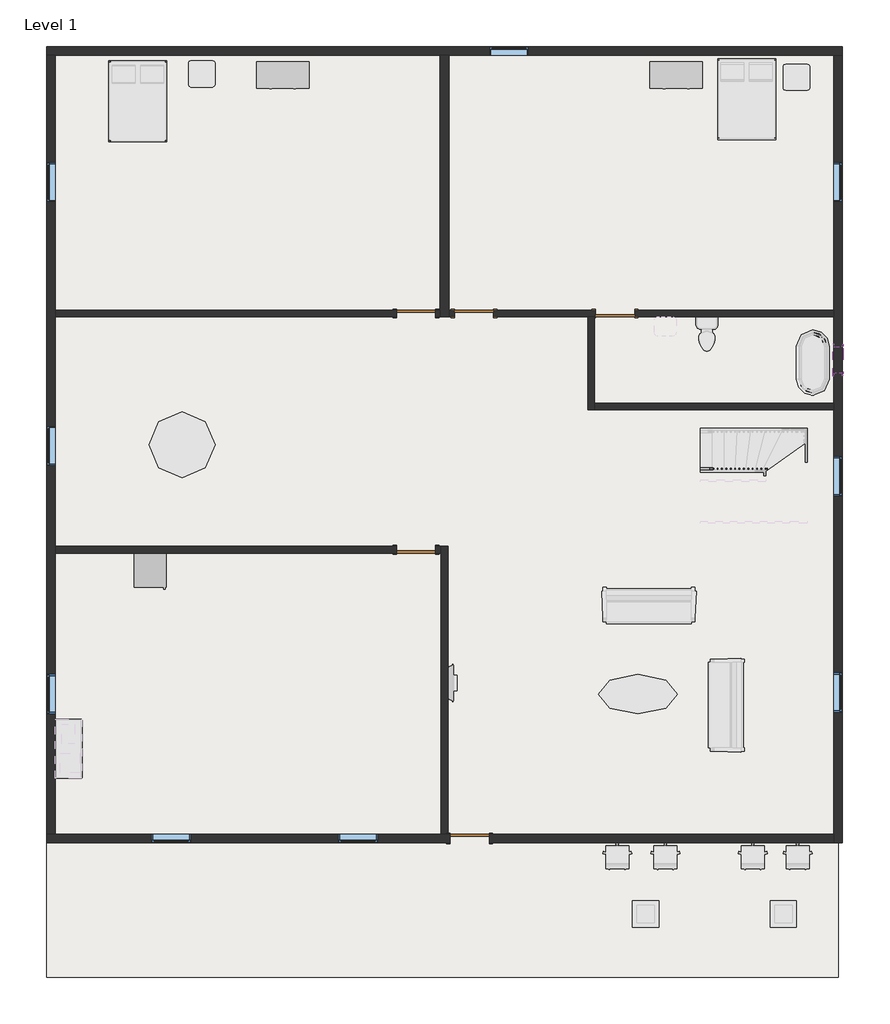
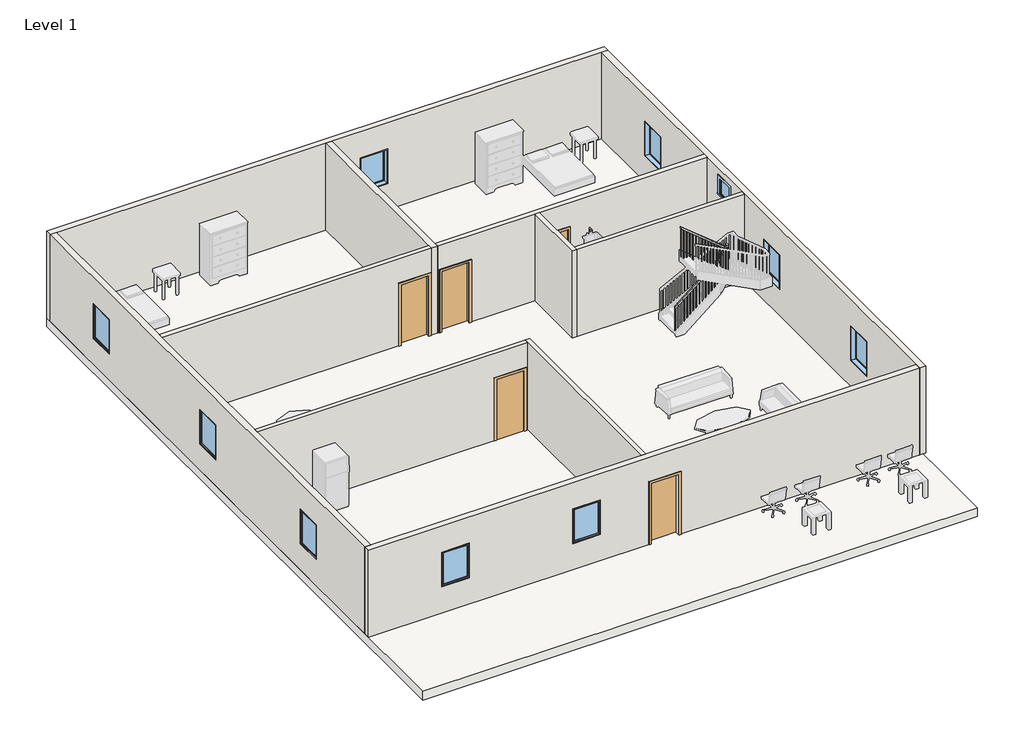
# One storey, part 1 of 2: 11 walls, 10 windows, 5 doors, 1 railing, 1 slab.
"""IFC4 building model written with IfcOpenShell, lengths in millimetres."""

from ifc_helpers import new_model, si_unit, frame, origin, origin_with_axes, place, context, project, spatial, polyline, outline, extrude, faceted_brep, transform, mapped, element, save
from components import door_16372e1c, door_686f89d2, door_719f80de, window_e2841890, window_e41d21a6

model = new_model("IFC4")

# Units and contexts
model_context = context("Model", 3, world=origin())
ifc_project = project(units=[si_unit("LENGTHUNIT", "METRE", prefix="MILLI")], contexts=[model_context])

# Site, building, storey
site = spatial("IfcSite", under=ifc_project)
building = spatial("IfcBuilding", under=site)
storey = spatial("IfcBuildingStorey", under=building, Name="Level 1", Elevation=0.0)

# Doors
placement = place(None, origin())
door_shape = door_16372e1c(model_context)
element("IfcDoor", 1, ObjectType="Single-Flush : 36\" x 84\"", at=placement, inside=storey, context=model_context, shape_type="MappedRepresentation", body=[
    mapped(door_shape, transform((-8051.9808972, 8246.1716937, 0.0), x_axis=(1.0, 0.0, 0.0), y_axis=(0.0, 1.0, 0.0), z_axis=(0.0, 0.0, 1.0))),
])
element("IfcDoor", 2, ObjectType="Single-Flush : 36\" x 84\"", at=placement, inside=storey, context=model_context, shape_type="MappedRepresentation", body=[
    mapped(door_shape, transform((-3429.1808972, 8246.1716937, 0.0), x_axis=(-1.0, 0.0, 0.0), y_axis=(0.0, -1.0, 0.0), z_axis=(0.0, 0.0, 1.0))),
])
door_2_shape = door_686f89d2(model_context)
element("IfcDoor", 3, ObjectType="Single-Flush : 36\" x 84\"", at=placement, inside=storey, context=model_context, shape_type="MappedRepresentation", body=[
    mapped(door_2_shape, transform((-6705.7808972, 8246.1716937, 0.0), x_axis=(-1.0, 0.0, 0.0), y_axis=(0.0, -1.0, 0.0), z_axis=(0.0, 0.0, 1.0))),
])
element("IfcDoor", 4, ObjectType="Single-Flush : 36\" x 84\"", at=placement, inside=storey, context=model_context, shape_type="MappedRepresentation", body=[
    mapped(door_2_shape, transform((-8051.9808972, 2759.7716937, 0.0), x_axis=(1.0, 0.0, 0.0), y_axis=(0.0, 1.0, 0.0), z_axis=(0.0, 0.0, 1.0))),
])
door_3_shape = door_719f80de(model_context)
element("IfcDoor", 5, ObjectType="Single-Flush : 36\" x 84\"", at=placement, inside=storey, context=model_context, shape_type="MappedRepresentation", body=[
    mapped(door_3_shape, transform((-6807.3808972, -3945.8283063, 0.0), x_axis=(-1.0, 0.0, 0.0), y_axis=(0.0, -1.0, 0.0), z_axis=(0.0, 0.0, 1.0))),
])

# Railing
element("IfcRailing", 6, ObjectType="Handrail - Rectangular", at=placement, inside=storey, context=model_context, shape_type="SolidModel", body=[
    faceted_brep([(-1451.7125891, 4664.7716937, 1025.2529681), (-1451.7125891, 4664.7716937, 959.7067088), (-1451.7125891, 4613.9716937, 959.7067088), (-1451.7125891, 4613.9716937, 1025.2529681), (-0.1808972, 4664.7716937, 2208.7848338), (50.6191028, 4664.7716937, 2184.659247), (50.6191028, 4613.9716937, 2184.659247), (-0.1808972, 4613.9716937, 2208.7848338), (-0.1808972, 4664.7716937, 2414.6281882), (50.6191028, 4664.7716937, 2363.8281882), (50.6191028, 4613.9716937, 2363.8281882), (-0.1808972, 4613.9716937, 2414.6281882), (126.8191028, 4664.7716937, 2414.6281882), (126.8191028, 4664.7716937, 2363.8281882), (76.0191028, 4613.9716937, 2363.8281882), (76.0191028, 4613.9716937, 2414.6281882), (126.8191028, 4537.7716937, 2414.6281882), (126.8191028, 4508.6503599, 2363.8281882), (76.0191028, 4508.6503599, 2363.8281882), (76.0191028, 4537.7716937, 2414.6281882), (126.8191028, 4410.7716937, 2631.5051451), (126.8191028, 4359.9716937, 2617.7256424), (76.0191028, 4359.9716937, 2617.7256424), (76.0191028, 4410.7716937, 2631.5051451), (126.8191028, 4410.7716937, 2837.3484995), (126.8191028, 4359.9716937, 2786.5484995), (76.0191028, 4359.9716937, 2786.5484995), (76.0191028, 4410.7716937, 2837.3484995), (126.8191028, 4283.7716937, 2837.3484995), (126.8191028, 4283.7716937, 2786.5484995), (76.0191028, 4334.5716937, 2786.5484995), (76.0191028, 4334.5716937, 2837.3484995), (-0.1808972, 4283.7716937, 2837.3484995), (-18.2663103, 4283.7716937, 2786.5484995), (-18.2663103, 4334.5716937, 2786.5484995), (-0.1808972, 4334.5716937, 2837.3484995), (-1451.7125891, 4283.7716937, 4020.8803652), (-1451.7125891, 4334.5716937, 4020.8803652), (-1451.7125891, 4334.5716937, 3955.3341059), (-1451.7125891, 4283.7716937, 3955.3341059)], [[[0, 1, 2, 3]], [[1, 0, 4, 5]], [[2, 1, 5, 6]], [[3, 2, 6, 7]], [[0, 3, 7, 4]], [[5, 4, 8, 9]], [[6, 5, 9, 10]], [[7, 6, 10, 11]], [[4, 7, 11, 8]], [[9, 8, 12, 13]], [[10, 9, 13, 14]], [[11, 10, 14, 15]], [[8, 11, 15, 12]], [[13, 12, 16, 17]], [[14, 13, 17, 18]], [[15, 14, 18, 19]], [[12, 15, 19, 16]], [[17, 16, 20, 21]], [[18, 17, 21, 22]], [[19, 18, 22, 23]], [[16, 19, 23, 20]], [[21, 20, 24, 25]], [[22, 21, 25, 26]], [[23, 22, 26, 27]], [[20, 23, 27, 24]], [[25, 24, 28, 29]], [[26, 25, 29, 30]], [[27, 26, 30, 31]], [[24, 27, 31, 28]], [[29, 28, 32, 33]], [[30, 29, 33, 34]], [[31, 30, 34, 35]], [[28, 31, 35, 32]], [[36, 37, 38, 39]], [[33, 32, 36, 39]], [[34, 33, 39, 38]], [[35, 34, 38, 37]], [[32, 35, 37, 36]]]),
    extrude(outline(polyline([(3866.2231262, -1342.4232536), (3881.7558784, -1361.4732536), (2878.6666667, -1361.4732536), (2878.6666667, -1342.4232536), (3866.2231262, -1342.4232536)])), frame((0.0, 4299.6466937, 0.0), z_axis=(0.0, 1.0, 0.0), x_axis=(0.0, 0.0, 1.0)), (0.0, 0.0, 1.0), 19.05),
    extrude(outline(polyline([(3783.3817813, -1240.8232536), (3798.9145334, -1259.8732536), (2878.6666667, -1259.8732536), (2878.6666667, -1240.8232536), (3783.3817813, -1240.8232536)])), frame((0.0, 4299.6466937, 0.0), z_axis=(0.0, 1.0, 0.0), x_axis=(0.0, 0.0, 1.0)), (0.0, 0.0, 1.0), 19.05),
    extrude(outline(polyline([(3700.5404364, -1139.2232536), (3716.0731885, -1158.2732536), (2709.3333333, -1158.2732536), (2709.3333333, -1139.2232536), (3700.5404364, -1139.2232536)])), frame((0.0, 4299.6466937, 0.0), z_axis=(0.0, 1.0, 0.0), x_axis=(0.0, 0.0, 1.0)), (0.0, 0.0, 1.0), 19.05),
    extrude(outline(polyline([(3617.6990914, -1037.6232536), (3633.2318436, -1056.6732536), (2709.3333333, -1056.6732536), (2709.3333333, -1037.6232536), (3617.6990914, -1037.6232536)])), frame((0.0, 4299.6466937, 0.0), z_axis=(0.0, 1.0, 0.0), x_axis=(0.0, 0.0, 1.0)), (0.0, 0.0, 1.0), 19.05),
    extrude(outline(polyline([(3534.8577465, -936.0232536), (3550.3904987, -955.0732536), (2709.3333333, -955.0732536), (2709.3333333, -936.0232536), (3534.8577465, -936.0232536)])), frame((0.0, 4299.6466937, 0.0), z_axis=(0.0, 1.0, 0.0), x_axis=(0.0, 0.0, 1.0)), (0.0, 0.0, 1.0), 19.05),
    extrude(outline(polyline([(3452.0164016, -834.4232536), (3467.5491538, -853.4732536), (2540.0, -853.4732536), (2540.0, -834.4232536), (3452.0164016, -834.4232536)])), frame((0.0, 4299.6466937, 0.0), z_axis=(0.0, 1.0, 0.0), x_axis=(0.0, 0.0, 1.0)), (0.0, 0.0, 1.0), 19.05),
    extrude(outline(polyline([(3369.1750567, -732.8232536), (3384.7078088, -751.8732536), (2540.0, -751.8732536), (2540.0, -732.8232536), (3369.1750567, -732.8232536)])), frame((0.0, 4299.6466937, 0.0), z_axis=(0.0, 1.0, 0.0), x_axis=(0.0, 0.0, 1.0)), (0.0, 0.0, 1.0), 19.05),
    extrude(outline(polyline([(3286.3337117, -631.2232536), (3301.8664639, -650.2732536), (2540.0, -650.2732536), (2540.0, -631.2232536), (3286.3337117, -631.2232536)])), frame((0.0, 4299.6466937, 0.0), z_axis=(0.0, 1.0, 0.0), x_axis=(0.0, 0.0, 1.0)), (0.0, 0.0, 1.0), 19.05),
    extrude(outline(polyline([(3203.4923668, -529.6232536), (3219.025119, -548.6732536), (2370.6666667, -548.6732536), (2370.6666667, -529.6232536), (3203.4923668, -529.6232536)])), frame((0.0, 4299.6466937, 0.0), z_axis=(0.0, 1.0, 0.0), x_axis=(0.0, 0.0, 1.0)), (0.0, 0.0, 1.0), 19.05),
    extrude(outline(polyline([(3120.6510219, -428.0232536), (3136.1837741, -447.0732536), (2370.6666667, -447.0732536), (2370.6666667, -428.0232536), (3120.6510219, -428.0232536)])), frame((0.0, 4299.6466937, 0.0), z_axis=(0.0, 1.0, 0.0), x_axis=(0.0, 0.0, 1.0)), (0.0, 0.0, 1.0), 19.05),
    extrude(outline(polyline([(3037.809677, -326.4232536), (3053.3424291, -345.4732536), (2201.3333333, -345.4732536), (2201.3333333, -326.4232536), (3037.809677, -326.4232536)])), frame((0.0, 4299.6466937, 0.0), z_axis=(0.0, 1.0, 0.0), x_axis=(0.0, 0.0, 1.0)), (0.0, 0.0, 1.0), 19.05),
    extrude(outline(polyline([(2954.9683321, -224.8232536), (2970.5010842, -243.8732536), (2201.3333333, -243.8732536), (2201.3333333, -224.8232536), (2954.9683321, -224.8232536)])), frame((0.0, 4299.6466937, 0.0), z_axis=(0.0, 1.0, 0.0), x_axis=(0.0, 0.0, 1.0)), (0.0, 0.0, 1.0), 19.05),
    extrude(outline(polyline([(2872.1269871, -123.2232536), (2887.6597393, -142.2732536), (2032.0, -142.2732536), (2032.0, -123.2232536), (2872.1269871, -123.2232536)])), frame((0.0, 4299.6466937, 0.0), z_axis=(0.0, 1.0, 0.0), x_axis=(0.0, 0.0, 1.0)), (0.0, 0.0, 1.0), 19.05),
    extrude(outline(polyline([(2789.2856422, -21.6232536), (2804.8183944, -40.6732536), (2032.0, -40.6732536), (2032.0, -21.6232536), (2789.2856422, -21.6232536)])), frame((0.0, 4299.6466937, 0.0), z_axis=(0.0, 1.0, 0.0), x_axis=(0.0, 0.0, 1.0)), (0.0, 0.0, 1.0), 19.05),
    extrude(outline(polyline([(4411.86079, 2529.115018), (4430.91079, 2496.5834745), (4430.91079, 1524.0), (4411.86079, 1524.0), (4411.86079, 2529.115018)])), frame((91.8941028, 0.0, 0.0), z_axis=(1.0, 0.0, 0.0), x_axis=(0.0, 1.0, 0.0)), (0.0, 0.0, 1.0), 19.05),
    extrude(outline(polyline([(4513.46079, 2355.6134525), (4532.51079, 2323.0819089), (4532.51079, 1524.0), (4513.46079, 1524.0), (4513.46079, 2355.6134525)])), frame((91.8941028, 0.0, 0.0), z_axis=(1.0, 0.0, 0.0), x_axis=(0.0, 1.0, 0.0)), (0.0, 0.0, 1.0), 19.05),
    extrude(outline(polyline([(2127.2519138, -19.7875891), (2111.7191617, -38.8375891), (1016.0, -38.8375891), (1016.0, -19.7875891), (2127.2519138, -19.7875891)])), frame((0.0, 4629.8466937, 0.0), z_axis=(0.0, 1.0, 0.0), x_axis=(0.0, 0.0, 1.0)), (0.0, 0.0, 1.0), 19.05),
    extrude(outline(polyline([(2044.4105689, -121.3875891), (2028.8778167, -140.4375891), (1016.0, -140.4375891), (1016.0, -121.3875891), (2044.4105689, -121.3875891)])), frame((0.0, 4629.8466937, 0.0), z_axis=(0.0, 1.0, 0.0), x_axis=(0.0, 0.0, 1.0)), (0.0, 0.0, 1.0), 19.05),
    extrude(outline(polyline([(1961.569224, -222.9875891), (1946.0364718, -242.0375891), (846.6666667, -242.0375891), (846.6666667, -222.9875891), (1961.569224, -222.9875891)])), frame((0.0, 4629.8466937, 0.0), z_axis=(0.0, 1.0, 0.0), x_axis=(0.0, 0.0, 1.0)), (0.0, 0.0, 1.0), 19.05),
    extrude(outline(polyline([(1878.7278791, -324.5875891), (1863.1951269, -343.6375891), (846.6666667, -343.6375891), (846.6666667, -324.5875891), (1878.7278791, -324.5875891)])), frame((0.0, 4629.8466937, 0.0), z_axis=(0.0, 1.0, 0.0), x_axis=(0.0, 0.0, 1.0)), (0.0, 0.0, 1.0), 19.05),
    extrude(outline(polyline([(1795.8865341, -426.1875891), (1780.353782, -445.2375891), (677.3333333, -445.2375891), (677.3333333, -426.1875891), (1795.8865341, -426.1875891)])), frame((0.0, 4629.8466937, 0.0), z_axis=(0.0, 1.0, 0.0), x_axis=(0.0, 0.0, 1.0)), (0.0, 0.0, 1.0), 19.05),
    extrude(outline(polyline([(1713.0451892, -527.7875891), (1697.5124371, -546.8375891), (677.3333333, -546.8375891), (677.3333333, -527.7875891), (1713.0451892, -527.7875891)])), frame((0.0, 4629.8466937, 0.0), z_axis=(0.0, 1.0, 0.0), x_axis=(0.0, 0.0, 1.0)), (0.0, 0.0, 1.0), 19.05),
    extrude(outline(polyline([(1630.2038443, -629.3875891), (1614.6710921, -648.4375891), (508.0, -648.4375891), (508.0, -629.3875891), (1630.2038443, -629.3875891)])), frame((0.0, 4629.8466937, 0.0), z_axis=(0.0, 1.0, 0.0), x_axis=(0.0, 0.0, 1.0)), (0.0, 0.0, 1.0), 19.05),
    extrude(outline(polyline([(1547.3624994, -730.9875891), (1531.8297472, -750.0375891), (508.0, -750.0375891), (508.0, -730.9875891), (1547.3624994, -730.9875891)])), frame((0.0, 4629.8466937, 0.0), z_axis=(0.0, 1.0, 0.0), x_axis=(0.0, 0.0, 1.0)), (0.0, 0.0, 1.0), 19.05),
    extrude(outline(polyline([(1464.5211545, -832.5875891), (1448.9884023, -851.6375891), (508.0, -851.6375891), (508.0, -832.5875891), (1464.5211545, -832.5875891)])), frame((0.0, 4629.8466937, 0.0), z_axis=(0.0, 1.0, 0.0), x_axis=(0.0, 0.0, 1.0)), (0.0, 0.0, 1.0), 19.05),
    extrude(outline(polyline([(1381.6798095, -934.1875891), (1366.1470574, -953.2375891), (338.6666667, -953.2375891), (338.6666667, -934.1875891), (1381.6798095, -934.1875891)])), frame((0.0, 4629.8466937, 0.0), z_axis=(0.0, 1.0, 0.0), x_axis=(0.0, 0.0, 1.0)), (0.0, 0.0, 1.0), 19.05),
    extrude(outline(polyline([(1298.8384646, -1035.7875891), (1283.3057124, -1054.8375891), (338.6666667, -1054.8375891), (338.6666667, -1035.7875891), (1298.8384646, -1035.7875891)])), frame((0.0, 4629.8466937, 0.0), z_axis=(0.0, 1.0, 0.0), x_axis=(0.0, 0.0, 1.0)), (0.0, 0.0, 1.0), 19.05),
    extrude(outline(polyline([(1215.9971197, -1137.3875891), (1200.4643675, -1156.4375891), (338.6666667, -1156.4375891), (338.6666667, -1137.3875891), (1215.9971197, -1137.3875891)])), frame((0.0, 4629.8466937, 0.0), z_axis=(0.0, 1.0, 0.0), x_axis=(0.0, 0.0, 1.0)), (0.0, 0.0, 1.0), 19.05),
    extrude(outline(polyline([(1133.1557748, -1238.9875891), (1117.6230226, -1258.0375891), (169.3333333, -1258.0375891), (169.3333333, -1238.9875891), (1133.1557748, -1238.9875891)])), frame((0.0, 4629.8466937, 0.0), z_axis=(0.0, 1.0, 0.0), x_axis=(0.0, 0.0, 1.0)), (0.0, 0.0, 1.0), 19.05),
    extrude(outline(polyline([(1050.3144298, -1340.5875891), (1034.7816777, -1359.6375891), (169.3333333, -1359.6375891), (169.3333333, -1340.5875891), (1050.3144298, -1340.5875891)])), frame((0.0, 4629.8466937, 0.0), z_axis=(0.0, 1.0, 0.0), x_axis=(0.0, 0.0, 1.0)), (0.0, 0.0, 1.0), 19.05),
    extrude(outline(polyline([(79.9767464, 4318.6966937), (79.9767464, 4299.6466937), (60.9267464, 4299.6466937), (60.9267464, 4318.6966937), (79.9767464, 4318.6966937)])), frame((0.0, 0.0, 1862.6666667), z_axis=(0.0, 0.0, 1.0), x_axis=(1.0, 0.0, 0.0)), (0.0, 0.0, 1.0), 923.8818329),
    extrude(outline(polyline([(91.8941028, 4318.6966937), (110.9441028, 4318.6966937), (110.9441028, 4299.6466937), (91.8941028, 4299.6466937), (91.8941028, 4318.6966937)])), frame((0.0, 0.0, 1862.6666667), z_axis=(0.0, 0.0, 1.0), x_axis=(1.0, 0.0, 0.0)), (0.0, 0.0, 1.0), 923.8818329),
    extrude(outline(polyline([(91.8941028, 4333.4825975), (110.9441028, 4333.4825975), (110.9441028, 4314.4325975), (91.8941028, 4314.4325975), (91.8941028, 4333.4825975)])), frame((0.0, 0.0, 1693.3333333), z_axis=(0.0, 0.0, 1.0), x_axis=(1.0, 0.0, 0.0)), (0.0, 0.0, 1.0), 1093.2151662),
    extrude(outline(polyline([(91.8941028, 4634.11079), (110.9441028, 4634.11079), (110.9441028, 4615.06079), (91.8941028, 4615.06079), (91.8941028, 4634.11079)])), frame((0.0, 0.0, 1354.6666667), z_axis=(0.0, 0.0, 1.0), x_axis=(1.0, 0.0, 0.0)), (0.0, 0.0, 1.0), 1009.1615215),
    extrude(outline(polyline([(91.8941028, 4629.8466937), (91.8941028, 4648.8966937), (110.9441028, 4648.8966937), (110.9441028, 4629.8466937), (91.8941028, 4629.8466937)])), frame((0.0, 0.0, 1185.3333333), z_axis=(0.0, 0.0, 1.0), x_axis=(1.0, 0.0, 0.0)), (0.0, 0.0, 1.0), 1178.4948549),
    extrude(outline(polyline([(60.9267464, 4629.8466937), (60.9267464, 4648.8966937), (79.9767464, 4648.8966937), (79.9767464, 4629.8466937), (60.9267464, 4629.8466937)])), frame((0.0, 0.0, 1185.3333333), z_axis=(0.0, 0.0, 1.0), x_axis=(1.0, 0.0, 0.0)), (0.0, 0.0, 1.0), 1178.4948549),
    extrude(outline(polyline([(3939.8013537, -1432.6625891), (3955.3341059, -1451.7125891), (2878.6666667, -1451.7125891), (2878.6666667, -1432.6625891), (3939.8013537, -1432.6625891)])), frame((0.0, 4299.6466937, 0.0), z_axis=(0.0, 1.0, 0.0), x_axis=(0.0, 0.0, 1.0)), (0.0, 0.0, 1.0), 19.05),
    extrude(outline(polyline([(975.239461, -1432.6625891), (959.7067088, -1451.7125891), (169.3333333, -1451.7125891), (169.3333333, -1432.6625891), (975.239461, -1432.6625891)])), frame((0.0, 4629.8466937, 0.0), z_axis=(0.0, 1.0, 0.0), x_axis=(0.0, 0.0, 1.0)), (0.0, 0.0, 1.0), 19.05),
])

# Slab
element("IfcSlab", 7, ObjectType="Generic - 12\"", at=placement, inside=storey, context=model_context, shape_type="SweptSolid", body=[
    extrude(outline(polyline([(1761.9441028, 14443.7716937), (1761.9441028, -7171.6283063), (-16637.1808972, -7171.6283063), (-16637.1808972, 14443.7716937), (1761.9441028, 14443.7716937)])), frame((0.0, 0.0, -304.8), z_axis=(0.0, 0.0, 1.0), x_axis=(1.0, 0.0, 0.0)), (0.0, 0.0, 1.0), 304.8),
])

# Walls
element("IfcWall", 8, ObjectType="Generic - 8\"", at=placement, inside=storey, context=model_context, shape_type="Brep", body=[
    faceted_brep([(-16637.1808972, 14240.5716937, 0.0), (-16433.9808972, 14240.5716937, 0.0), (-7493.1808972, 14240.5716937, 0.0), (-7289.9808972, 14240.5716937, 0.0), (1650.8191028, 14240.5716937, 0.0), (1854.0191028, 14240.5716937, 0.0), (1854.0191028, 14240.5716937, 3048.0), (1650.8191028, 14240.5716937, 3048.0), (-7289.9808972, 14240.5716937, 3048.0), (-7493.1808972, 14240.5716937, 3048.0), (-16433.9808972, 14240.5716937, 3048.0), (-16637.1808972, 14240.5716937, 3048.0), (-5435.7808972, 14240.5716937, 2133.6), (-5435.7808972, 14240.5716937, 914.4), (-6350.1808972, 14240.5716937, 914.4), (-6350.1808972, 14240.5716937, 2133.6), (-16637.1808972, 14443.7716937, 0.0), (-16637.1808972, 14443.7716937, 3048.0), (1854.0191028, 14443.7716937, 3048.0), (1854.0191028, 14443.7716937, 0.0), (-5435.7808972, 14443.7716937, 2133.6), (-6350.1808972, 14443.7716937, 2133.6), (-6350.1808972, 14443.7716937, 914.4), (-5435.7808972, 14443.7716937, 914.4)], [[[0, 1, 2, 3, 4, 5, 6, 7, 8, 9, 10, 11], [12, 13, 14, 15]], [[16, 17, 18, 19], [20, 21, 22, 23]], [[5, 4, 3, 2, 1, 0, 16, 19]], [[11, 10, 9, 8, 7, 6, 18, 17]], [[6, 5, 19, 18]], [[0, 11, 17, 16]], [[13, 12, 20, 23]], [[14, 13, 23, 22]], [[15, 14, 22, 21]], [[12, 15, 21, 20]]]),
])
element("IfcWall", 9, ObjectType="Generic - 8\"", at=placement, inside=storey, context=model_context, shape_type="Brep", body=[
    faceted_brep([(1650.8191028, 14240.5716937, 0.0), (1650.8191028, 8322.3716937, 0.0), (1650.8191028, 8169.9716937, 0.0), (1650.8191028, 6163.3716937, 0.0), (1650.8191028, 6010.9716937, 0.0), (1650.8191028, -3844.2283063, 0.0), (1650.8191028, -4047.4283063, 0.0), (1650.8191028, -4047.4283063, 3048.0), (1650.8191028, -3844.2283063, 3048.0), (1650.8191028, 6010.9716937, 3048.0), (1650.8191028, 6163.3716937, 3048.0), (1650.8191028, 8169.9716937, 3048.0), (1650.8191028, 8322.3716937, 3048.0), (1650.8191028, 14240.5716937, 3048.0), (1650.8191028, -1008.9533063, 2133.6), (1650.8191028, -1008.9533063, 914.4), (1650.8191028, -94.5533063, 914.4), (1650.8191028, -94.5533063, 2133.6), (1650.8191028, 4007.5466937, 2133.6), (1650.8191028, 4007.5466937, 914.4), (1650.8191028, 4921.9466937, 914.4), (1650.8191028, 4921.9466937, 2133.6), (1650.8191028, 10836.9716937, 2133.6), (1650.8191028, 10836.9716937, 914.4), (1650.8191028, 11751.3716937, 914.4), (1650.8191028, 11751.3716937, 2133.6), (1650.8191028, 7471.4716937, 2768.6), (1650.8191028, 6861.8716937, 2768.6), (1650.8191028, 6861.8716937, 2159.0), (1650.8191028, 7471.4716937, 2159.0), (1854.0191028, 14240.5716937, 0.0), (1854.0191028, 14240.5716937, 3048.0), (1854.0191028, -4047.4283063, 3048.0), (1854.0191028, -4047.4283063, 0.0), (1854.0191028, -1008.9533063, 2133.6), (1854.0191028, -94.5533063, 2133.6), (1854.0191028, -94.5533063, 914.4), (1854.0191028, -1008.9533063, 914.4), (1854.0191028, 4007.5466937, 2133.6), (1854.0191028, 4921.9466937, 2133.6), (1854.0191028, 4921.9466937, 914.4), (1854.0191028, 4007.5466937, 914.4), (1854.0191028, 10836.9716937, 2133.6), (1854.0191028, 11751.3716937, 2133.6), (1854.0191028, 11751.3716937, 914.4), (1854.0191028, 10836.9716937, 914.4), (1854.0191028, 7471.4716937, 2768.6), (1854.0191028, 7471.4716937, 2159.0), (1854.0191028, 6861.8716937, 2159.0), (1854.0191028, 6861.8716937, 2768.6)], [[[0, 1, 2, 3, 4, 5, 6, 7, 8, 9, 10, 11, 12, 13], [14, 15, 16, 17], [18, 19, 20, 21], [22, 23, 24, 25], [26, 27, 28, 29]], [[30, 31, 32, 33], [34, 35, 36, 37], [38, 39, 40, 41], [42, 43, 44, 45], [46, 47, 48, 49]], [[6, 5, 4, 3, 2, 1, 0, 30, 33]], [[13, 12, 11, 10, 9, 8, 7, 32, 31]], [[0, 13, 31, 30]], [[7, 6, 33, 32]], [[15, 14, 34, 37]], [[16, 15, 37, 36]], [[17, 16, 36, 35]], [[14, 17, 35, 34]], [[19, 18, 38, 41]], [[20, 19, 41, 40]], [[21, 20, 40, 39]], [[18, 21, 39, 38]], [[23, 22, 42, 45]], [[24, 23, 45, 44]], [[25, 24, 44, 43]], [[22, 25, 43, 42]], [[47, 46, 26, 29]], [[48, 47, 29, 28]], [[49, 48, 28, 27]], [[46, 49, 27, 26]]]),
])
element("IfcWall", 10, ObjectType="Generic - 8\"", at=placement, inside=storey, context=model_context, shape_type="Brep", body=[
    faceted_brep([(-7264.5808972, -3844.2283063, 2133.6), (-7264.5808972, -3844.2283063, 0.0), (-7315.3808972, -3844.2283063, 0.0), (-7467.7808972, -3844.2283063, 0.0), (-16433.9808972, -3844.2283063, 0.0), (-16637.1808972, -3844.2283063, 0.0), (-16637.1808972, -3844.2283063, 3048.0), (-16433.9808972, -3844.2283063, 3048.0), (-7467.7808972, -3844.2283063, 3048.0), (-7315.3808972, -3844.2283063, 3048.0), (1650.8191028, -3844.2283063, 3048.0), (1650.8191028, -3844.2283063, 0.0), (-6350.1808972, -3844.2283063, 0.0), (-6350.1808972, -3844.2283063, 2133.6), (-14198.7808972, -3844.2283063, 2133.6), (-14198.7808972, -3844.2283063, 914.4), (-13284.3808972, -3844.2283063, 914.4), (-13284.3808972, -3844.2283063, 2133.6), (-9855.3808972, -3844.2283063, 2133.6), (-9855.3808972, -3844.2283063, 914.4), (-8940.9808972, -3844.2283063, 914.4), (-8940.9808972, -3844.2283063, 2133.6), (-16637.1808972, -4047.4283063, 0.0), (-7264.5808972, -4047.4283063, 0.0), (-7264.5808972, -4047.4283063, 2133.6), (-6350.1808972, -4047.4283063, 2133.6), (-6350.1808972, -4047.4283063, 0.0), (1650.8191028, -4047.4283063, 0.0), (1650.8191028, -4047.4283063, 3048.0), (-16637.1808972, -4047.4283063, 3048.0), (-14198.7808972, -4047.4283063, 2133.6), (-13284.3808972, -4047.4283063, 2133.6), (-13284.3808972, -4047.4283063, 914.4), (-14198.7808972, -4047.4283063, 914.4), (-9855.3808972, -4047.4283063, 2133.6), (-8940.9808972, -4047.4283063, 2133.6), (-8940.9808972, -4047.4283063, 914.4), (-9855.3808972, -4047.4283063, 914.4)], [[[0, 1, 2, 3, 4, 5, 6, 7, 8, 9, 10, 11, 12, 13], [14, 15, 16, 17], [18, 19, 20, 21]], [[22, 23, 24, 25, 26, 27, 28, 29], [30, 31, 32, 33], [34, 35, 36, 37]], [[12, 11, 27, 26]], [[5, 4, 3, 2, 1, 23, 22]], [[10, 9, 8, 7, 6, 29, 28]], [[11, 10, 28, 27]], [[6, 5, 22, 29]], [[24, 23, 1, 0]], [[25, 24, 0, 13]], [[26, 25, 13, 12]], [[15, 14, 30, 33]], [[16, 15, 33, 32]], [[17, 16, 32, 31]], [[14, 17, 31, 30]], [[19, 18, 34, 37]], [[20, 19, 37, 36]], [[21, 20, 36, 35]], [[18, 21, 35, 34]]]),
])
element("IfcWall", 11, ObjectType="Generic - 8\"", at=placement, inside=storey, context=model_context, shape_type="Brep", body=[
    faceted_brep([(-16433.9808972, -3844.2283063, 0.0), (-16433.9808972, 2683.5716937, 0.0), (-16433.9808972, 2835.9716937, 0.0), (-16433.9808972, 8169.9716937, 0.0), (-16433.9808972, 8322.3716937, 0.0), (-16433.9808972, 14240.5716937, 0.0), (-16433.9808972, 14240.5716937, 3048.0), (-16433.9808972, 8322.3716937, 3048.0), (-16433.9808972, 8169.9716937, 3048.0), (-16433.9808972, 2835.9716937, 3048.0), (-16433.9808972, 2683.5716937, 3048.0), (-16433.9808972, -3844.2283063, 3048.0), (-16433.9808972, 11751.3716937, 2133.6), (-16433.9808972, 11751.3716937, 914.4), (-16433.9808972, 10836.9716937, 914.4), (-16433.9808972, 10836.9716937, 2133.6), (-16433.9808972, 5629.9716937, 2133.6), (-16433.9808972, 5629.9716937, 914.4), (-16433.9808972, 4715.5716937, 914.4), (-16433.9808972, 4715.5716937, 2133.6), (-16433.9808972, -135.8283063, 2133.6), (-16433.9808972, -135.8283063, 914.4), (-16433.9808972, -1050.2283063, 914.4), (-16433.9808972, -1050.2283063, 2133.6), (-16637.1808972, -3844.2283063, 0.0), (-16637.1808972, -3844.2283063, 3048.0), (-16637.1808972, 14240.5716937, 3048.0), (-16637.1808972, 14240.5716937, 0.0), (-16637.1808972, 11751.3716937, 2133.6), (-16637.1808972, 10836.9716937, 2133.6), (-16637.1808972, 10836.9716937, 914.4), (-16637.1808972, 11751.3716937, 914.4), (-16637.1808972, 5629.9716937, 2133.6), (-16637.1808972, 4715.5716937, 2133.6), (-16637.1808972, 4715.5716937, 914.4), (-16637.1808972, 5629.9716937, 914.4), (-16637.1808972, -135.8283063, 2133.6), (-16637.1808972, -1050.2283063, 2133.6), (-16637.1808972, -1050.2283063, 914.4), (-16637.1808972, -135.8283063, 914.4)], [[[0, 1, 2, 3, 4, 5, 6, 7, 8, 9, 10, 11], [12, 13, 14, 15], [16, 17, 18, 19], [20, 21, 22, 23]], [[24, 25, 26, 27], [28, 29, 30, 31], [32, 33, 34, 35], [36, 37, 38, 39]], [[5, 4, 3, 2, 1, 0, 24, 27]], [[11, 10, 9, 8, 7, 6, 26, 25]], [[6, 5, 27, 26]], [[0, 11, 25, 24]], [[13, 12, 28, 31]], [[14, 13, 31, 30]], [[15, 14, 30, 29]], [[12, 15, 29, 28]], [[17, 16, 32, 35]], [[18, 17, 35, 34]], [[19, 18, 34, 33]], [[16, 19, 33, 32]], [[21, 20, 36, 39]], [[22, 21, 39, 38]], [[23, 22, 38, 37]], [[20, 23, 37, 36]]]),
])
element("IfcWall", 12, ObjectType="Generic - 8\"", at=placement, inside=storey, context=model_context, shape_type="Brep", body=[
    faceted_brep([(-7493.1808972, 14240.5716937, 0.0), (-7493.1808972, 8322.3716937, 0.0), (-7493.1808972, 8169.9716937, 0.0), (-7493.1808972, 8169.9716937, 3048.0), (-7493.1808972, 8322.3716937, 3048.0), (-7493.1808972, 14240.5716937, 3048.0), (-7289.9808972, 14240.5716937, 0.0), (-7289.9808972, 14240.5716937, 3048.0), (-7289.9808972, 8322.3716937, 3048.0), (-7289.9808972, 8169.9716937, 3048.0), (-7289.9808972, 8169.9716937, 0.0), (-7289.9808972, 8322.3716937, 0.0)], [[[0, 1, 2, 3, 4, 5]], [[6, 7, 8, 9, 10, 11]], [[2, 1, 0, 6, 11, 10]], [[5, 4, 3, 9, 8, 7]], [[0, 5, 7, 6]], [[3, 2, 10, 9]]]),
])
element("IfcWall", 13, ObjectType="inner wall", at=placement, inside=storey, context=model_context, shape_type="SweptSolid", body=[
    extrude(outline(polyline([(2133.6, -7594.7808972), (0.0, -7594.7808972), (0.0, -7493.1808972), (3048.0, -7493.1808972), (3048.0, -16433.9808972), (0.0, -16433.9808972), (0.0, -8509.1808972), (2133.6, -8509.1808972), (2133.6, -7594.7808972)])), frame((0.0, 8169.9716937, 0.0), z_axis=(0.0, 1.0, 0.0), x_axis=(0.0, 0.0, 1.0)), (0.0, 0.0, 1.0), 152.4),
])
element("IfcWall", 14, ObjectType="inner wall", at=placement, inside=storey, context=model_context, shape_type="Brep", body=[
    faceted_brep([(-3886.3808972, 8322.3716937, 2133.6), (-3886.3808972, 8322.3716937, 0.0), (-6248.5808972, 8322.3716937, 0.0), (-6248.5808972, 8322.3716937, 2133.6), (-7162.9808972, 8322.3716937, 2133.6), (-7162.9808972, 8322.3716937, 0.0), (-7289.9808972, 8322.3716937, 0.0), (-7289.9808972, 8322.3716937, 3048.0), (1650.8191028, 8322.3716937, 3048.0), (1650.8191028, 8322.3716937, 0.0), (-2971.9808972, 8322.3716937, 0.0), (-2971.9808972, 8322.3716937, 2133.6), (-6248.5808972, 8169.9716937, 0.0), (-4064.1808972, 8169.9716937, 0.0), (-3911.7808972, 8169.9716937, 0.0), (-3886.3808972, 8169.9716937, 0.0), (-3886.3808972, 8169.9716937, 2133.6), (-2971.9808972, 8169.9716937, 2133.6), (-2971.9808972, 8169.9716937, 0.0), (1650.8191028, 8169.9716937, 0.0), (1650.8191028, 8169.9716937, 3048.0), (-3911.7808972, 8169.9716937, 3048.0), (-4064.1808972, 8169.9716937, 3048.0), (-7289.9808972, 8169.9716937, 3048.0), (-7289.9808972, 8169.9716937, 0.0), (-7162.9808972, 8169.9716937, 0.0), (-7162.9808972, 8169.9716937, 2133.6), (-6248.5808972, 8169.9716937, 2133.6)], [[[0, 1, 2, 3, 4, 5, 6, 7, 8, 9, 10, 11]], [[12, 13, 14, 15, 16, 17, 18, 19, 20, 21, 22, 23, 24, 25, 26, 27]], [[6, 5, 25, 24]], [[10, 9, 19, 18]], [[2, 1, 15, 14, 13, 12]], [[8, 7, 23, 22, 21, 20]], [[9, 8, 20, 19]], [[7, 6, 24, 23]], [[26, 25, 5, 4]], [[27, 26, 4, 3]], [[12, 27, 3, 2]], [[16, 15, 1, 0]], [[17, 16, 0, 11]], [[18, 17, 11, 10]]]),
])
element("IfcWall", 15, ObjectType="inner wall", at=placement, inside=storey, context=model_context, shape_type="SweptSolid", body=[
    extrude(outline(polyline([(2133.6, -7594.7808972), (0.0, -7594.7808972), (0.0, -7467.7808972), (3048.0, -7467.7808972), (3048.0, -16433.9808972), (0.0, -16433.9808972), (0.0, -8509.1808972), (2133.6, -8509.1808972), (2133.6, -7594.7808972)])), frame((0.0, 2683.5716937, 0.0), z_axis=(0.0, 1.0, 0.0), x_axis=(0.0, 0.0, 1.0)), (0.0, 0.0, 1.0), 152.4),
])
element("IfcWall", 16, ObjectType="inner wall", at=placement, inside=storey, context=model_context, shape_type="Brep", body=[
    faceted_brep([(-4064.1808972, 8169.9716937, 0.0), (-4064.1808972, 6010.9716937, 0.0), (-4064.1808972, 6010.9716937, 3048.0), (-4064.1808972, 8169.9716937, 3048.0), (-3911.7808972, 8169.9716937, 0.0), (-3911.7808972, 8169.9716937, 3048.0), (-3911.7808972, 6163.3716937, 3048.0), (-3911.7808972, 6010.9716937, 3048.0), (-3911.7808972, 6010.9716937, 0.0), (-3911.7808972, 6163.3716937, 0.0)], [[[0, 1, 2, 3]], [[4, 5, 6, 7, 8, 9]], [[1, 0, 4, 9, 8]], [[3, 2, 7, 6, 5]], [[0, 3, 5, 4]], [[2, 1, 8, 7]]]),
])
element("IfcWall", 17, ObjectType="inner wall", at=placement, inside=storey, context=model_context, shape_type="SweptSolid", body=[
    extrude(outline(polyline([(1650.8191028, 6010.9716937), (-3911.7808972, 6010.9716937), (-3911.7808972, 6163.3716937), (1650.8191028, 6163.3716937), (1650.8191028, 6010.9716937)])), origin_with_axes(), (0.0, 0.0, 1.0), 3048.0),
])
element("IfcWall", 18, ObjectType="inner wall", at=placement, inside=storey, context=model_context, shape_type="Brep", body=[
    faceted_brep([(-7467.7808972, 2842.3216937, 0.0), (-7467.7808972, 2835.9716937, 0.0), (-7467.7808972, 2683.5716937, 0.0), (-7467.7808972, -3844.2283063, 0.0), (-7467.7808972, -3844.2283063, 3048.0), (-7467.7808972, 2683.5716937, 3048.0), (-7467.7808972, 2835.9716937, 3048.0), (-7467.7808972, 2842.3216937, 3048.0), (-7315.3808972, 2842.3216937, 0.0), (-7315.3808972, 2842.3216937, 3048.0), (-7315.3808972, -3844.2283063, 3048.0), (-7315.3808972, -3844.2283063, 0.0)], [[[0, 1, 2, 3, 4, 5, 6, 7]], [[8, 9, 10, 11]], [[3, 2, 1, 0, 8, 11]], [[7, 6, 5, 4, 10, 9]], [[0, 7, 9, 8]], [[4, 3, 11, 10]]]),
])

# Windows
window_shape = window_e2841890(model_context)
element("IfcWindow", 19, ObjectType="Fixed : 36\" x 48\"", at=placement, inside=storey, context=model_context, shape_type="MappedRepresentation", body=[
    mapped(window_shape, transform((-16535.5808972, 11332.2716937, 0.0), x_axis=(0.0, 1.0, 0.0), y_axis=(-1.0, 0.0, 0.0), z_axis=(0.0, 0.0, 1.0))),
])
element("IfcWindow", 20, ObjectType="Fixed : 36\" x 48\"", at=placement, inside=storey, context=model_context, shape_type="MappedRepresentation", body=[
    mapped(window_shape, transform((-16535.5808972, 5210.8716937, 0.0), x_axis=(0.0, 1.0, 0.0), y_axis=(-1.0, 0.0, 0.0), z_axis=(0.0, 0.0, 1.0))),
])
element("IfcWindow", 21, ObjectType="Fixed : 36\" x 48\"", at=placement, inside=storey, context=model_context, shape_type="MappedRepresentation", body=[
    mapped(window_shape, transform((-16535.5808972, -554.9283063, 0.0), x_axis=(0.0, 1.0, 0.0), y_axis=(-1.0, 0.0, 0.0), z_axis=(0.0, 0.0, 1.0))),
])
element("IfcWindow", 22, ObjectType="Fixed : 36\" x 48\"", at=placement, inside=storey, context=model_context, shape_type="MappedRepresentation", body=[
    mapped(window_shape, transform((-13779.6808972, -3945.8283063, 0.0), x_axis=(-1.0, 0.0, 0.0), y_axis=(0.0, -1.0, 0.0), z_axis=(0.0, 0.0, 1.0))),
])
element("IfcWindow", 23, ObjectType="Fixed : 36\" x 48\"", at=placement, inside=storey, context=model_context, shape_type="MappedRepresentation", body=[
    mapped(window_shape, transform((-9436.2808972, -3945.8283063, 0.0), x_axis=(-1.0, 0.0, 0.0), y_axis=(0.0, -1.0, 0.0), z_axis=(0.0, 0.0, 1.0))),
])
element("IfcWindow", 24, ObjectType="Fixed : 36\" x 48\"", at=placement, inside=storey, context=model_context, shape_type="MappedRepresentation", body=[
    mapped(window_shape, transform((1752.4191028, -589.8533063, 0.0), x_axis=(0.0, -1.0, 0.0), y_axis=(1.0, 0.0, 0.0), z_axis=(0.0, 0.0, 1.0))),
])
element("IfcWindow", 25, ObjectType="Fixed : 36\" x 48\"", at=placement, inside=storey, context=model_context, shape_type="MappedRepresentation", body=[
    mapped(window_shape, transform((1752.4191028, 4426.6466937, 0.0), x_axis=(0.0, -1.0, 0.0), y_axis=(1.0, 0.0, 0.0), z_axis=(0.0, 0.0, 1.0))),
])
element("IfcWindow", 26, ObjectType="Fixed : 36\" x 48\"", at=placement, inside=storey, context=model_context, shape_type="MappedRepresentation", body=[
    mapped(window_shape, transform((-5854.8808972, 14342.1716937, 0.0), x_axis=(1.0, 0.0, 0.0), y_axis=(0.0, 1.0, 0.0), z_axis=(0.0, 0.0, 1.0))),
])
element("IfcWindow", 27, ObjectType="Fixed : 36\" x 48\"", at=placement, inside=storey, context=model_context, shape_type="MappedRepresentation", body=[
    mapped(window_shape, transform((1752.4191028, 11256.0716937, 0.0), x_axis=(0.0, -1.0, 0.0), y_axis=(1.0, 0.0, 0.0), z_axis=(0.0, 0.0, 1.0))),
])
window_2_shape = window_e41d21a6(model_context)
element("IfcWindow", 28, ObjectType="Transom with Trim : 24\" x 24\"", at=placement, inside=storey, context=model_context, shape_type="MappedRepresentation", body=[
    mapped(window_2_shape, transform((1752.4191028, 7204.7716937, 0.0), x_axis=(0.0, 1.0, 0.0), y_axis=(-1.0, 0.0, 0.0), z_axis=(0.0, 0.0, 1.0))),
])

save(model, "model.ifc")

# Revit data of these elements
# Type "Single-Flush : 36\" x 84\""
#   Type Mark = "1"
#   Construction Type Id = "MDOOR"
#   Assembly Code = "C1020"
#   Analytic Construction = "Metal"
#   Thickness = 0' - 2"
#   Heat Transfer Coefficient (U) = 0.651978 BTU/(h·ft²·°F)
#   Height = 7' - 0"
#   Trim Projection Ext = 0' - 1"
#   Trim Projection Int = 0' - 1"
#   Trim Width = 0' - 3"
#   Width = 3' - 0"
#   Define Thermal Properties by = 1
#   Door Material = Door - Panel
#   Frame Material = Door - Frame
#   Visual Light Transmittance = 0
#   Solar Heat Gain Coefficient = 0
#   Function = (empty or 0)
#   Wall Closure = (empty or 0)
# Type "Handrail - Rectangular"
#   Assembly Code = "C2010400"
#   built-in parameter 1008612 = 0.0416667 (stored number, unit not read)
#   built-in parameter 1008611 = 0.0416667 (stored number, unit not read)
#   built-in parameter 1008609 = 0.333333 (stored number, unit not read)
#   built-in parameter 1008604 = 0.166667 (stored number, unit not read)
#   built-in parameter 1008603 = 0.166667 (stored number, unit not read)
#   Railing Height = 3' - 0"
#   built-in parameter 1008630 = 2
#   built-in parameter 1008610 = 2
#   built-in parameter 1008618 = Baluster - Square : 3/4"
# Type "Generic - 12\""
#   Assembly Code = "B1010"
#   Function = 0
#   Layers, outside or top first: 1' - 0" no material (function 1)
# Type "Generic - 8\""
#   Assembly Code = "B2010"
#   Layers, outside or top first: 0' - 8" "Brick, Common" (function 1)
# Type "inner wall"
#   Assembly Code = "B2010"
#   Layers, outside or top first: 0' - 6" "Brick, Common" (function 1)
# Type "Fixed : 36\" x 48\""
#   Type Mark = "1"
#   Construction Type Id = "GSP4R"
#   Assembly Code = "B2020100"
#   Analytic Construction = "1/8 in Pilkington single glazing"
#   Visual Light Transmittance = 0.9
#   Solar Heat Gain Coefficient = 0.78
#   Heat Transfer Coefficient (U) = 0.6496 BTU/(h·ft²·°F)
#   Height = 4' - 0"
#   Default Sill Height = 3' - 0"
#   Width = 3' - 0"
#   Window Inset = 0' - 0 3/4"
#   Define Thermal Properties by = 1
#   Glass Pane Material = Glass
#   Sash Material = Sash
#   Wall Closure = (empty or 0)
# Type "Transom with Trim : 24\" x 24\""
#   Type Mark = "10"
#   Construction Type Id = "GSP4R"
#   Assembly Code = "B2020100"
#   Analytic Construction = "1/8 in Pilkington single glazing"
#   Visual Light Transmittance = 0.9
#   Solar Heat Gain Coefficient = 0.78
#   Heat Transfer Coefficient (U) = 0.6496 BTU/(h·ft²·°F)
#   Height = 2' - 0"
#   Default Sill Height = 7' - 1"
#   Trim Projection - Ext. = 0' - 0 1/2"
#   Trim Projection - Int. = 0' - 0 3/4"
#   Trim Width - Exterior = 0' - 3 1/2"
#   Trim Width - Interior = 0' - 3 1/2"
#   Width = 2' - 0"
#   Window Inset = 0' - 0 3/4"
#   Define Thermal Properties by = 1
#   Glass Pane Material = Glass
#   Sash Material = Sash
#   Trim Exterior Material = Trim
#   Trim Interior Material = Trim
#   Wall Closure = (empty or 0)
# Elements 1, 2, 3, 4, 5 (IfcDoor, "Single-Flush : 36\" x 84\"")
#   Phase Created = New Construction
#   Materials on its faces: "Door - Frame", "Door - Panel"
# Element 6 (IfcRailing, "Handrail - Rectangular")
#   Phase Created = New Construction
# Element 7 (IfcSlab, "Generic - 12\"")
#   Height Offset From Level = 0' - 0"
#   Phase Created = New Construction
#   Materials on its faces: "Default Floor"
# Elements 8, 9, 10, 11, 12 (IfcWall, "Generic - 8\"")
#   Top Offset = 0' - 0"
#   Base Offset = 0' - 0"
#   Unconnected Height = 10' - 0"
#   wall height = 10' - 0"
#   Phase Created = New Construction
#   Base Constraint = Level 1
#   Materials on its faces: "Brick, Common"
# Elements 13, 14, 15, 16, 17, 18 (IfcWall, "inner wall")
#   Top Offset = 0' - 0"
#   Base Offset = 0' - 0"
#   Unconnected Height = 10' - 0"
#   wall height = 10' - 0"
#   Phase Created = New Construction
#   Base Constraint = Level 1
#   Materials on its faces: "Brick, Common"
# Element 19 (IfcWindow, "Fixed : 36\" x 48\"")
#   Mark = "1"
#   Phase Created = New Construction
#   Materials on its faces: "Sash", "Glass"
# Element 20 (IfcWindow, "Fixed : 36\" x 48\"")
#   Mark = "2"
#   Phase Created = New Construction
#   Materials on its faces: "Sash", "Glass"
# Element 21 (IfcWindow, "Fixed : 36\" x 48\"")
#   Mark = "3"
#   Phase Created = New Construction
#   Materials on its faces: "Sash", "Glass"
# Element 22 (IfcWindow, "Fixed : 36\" x 48\"")
#   Mark = "4"
#   Phase Created = New Construction
#   Materials on its faces: "Sash", "Glass"
# Element 23 (IfcWindow, "Fixed : 36\" x 48\"")
#   Mark = "5"
#   Phase Created = New Construction
#   Materials on its faces: "Sash", "Glass"
# Element 24 (IfcWindow, "Fixed : 36\" x 48\"")
#   Mark = "6"
#   Phase Created = New Construction
#   Materials on its faces: "Sash", "Glass"
# Element 25 (IfcWindow, "Fixed : 36\" x 48\"")
#   Mark = "7"
#   Phase Created = New Construction
#   Materials on its faces: "Sash", "Glass"
# Element 26 (IfcWindow, "Fixed : 36\" x 48\"")
#   Mark = "8"
#   Phase Created = New Construction
#   Materials on its faces: "Sash", "Glass"
# Element 27 (IfcWindow, "Fixed : 36\" x 48\"")
#   Mark = "9"
#   Phase Created = New Construction
#   Materials on its faces: "Sash", "Glass"
# Element 28 (IfcWindow, "Transom with Trim : 24\" x 24\"")
#   Mark = "10"
#   Phase Created = New Construction
#   Materials on its faces: "Sash", "Trim", "Glass"
# Materials
#   "Door - Panel": class "Wood", colour RGB 210 159 95, transparency 0
#   "Door - Frame": colour RGB 118 70 51, transparency 0
#   "Brick, Common": class "Masonry", colour RGB 170 98 104, transparency 0, Description = "Common brick", Cost = 0
#   "Glass": class "Glass", colour RGB 0 128 192, transparency 0.75, Description = "Soda Lime Glass", Cost = 0
#   "Sash": class "Wood", colour RGB 224 178 126, transparency 0
#   "Trim": class "Wood", colour RGB 224 178 126, transparency 0
#   "Default Floor": colour RGB 128 128 128, transparency 0
# Room at (-1963.982, 11047.346) mm, phase "New Construction", upper level "Level 1", upper offset 10' - 0", lower offset 0' - 0"
#   Number = "2"
#   Name = "BEDROOM"
# Room at (-1963.982, 7164.42) mm, phase "New Construction", upper level "Level 1", upper offset 10' - 0", lower offset 0' - 0"
#   Number = "4"
#   Name = "TOILET BATH"
# Room at (-11966.737, 11047.346) mm, phase "New Construction", upper level "Level 1", upper offset 10' - 0", lower offset 0' - 0"
#   Number = "1"
#   Name = "BED ROOM"
# Room at (-10137.937, 5349.574) mm, phase "New Construction", upper level "Level 1", upper offset 10' - 0", lower offset 0' - 0"
#   Number = "3"
#   Name = "DINING HALL"
# Room at (-11966.737, -643.638) mm, phase "New Construction", upper level "Level 1", upper offset 10' - 0", lower offset 0' - 0"
#   Number = "5"
#   Name = "KITCHEN"
# Room at (-3061.33, 0) mm, phase "New Construction", upper level "Level 1", upper offset 10' - 0", lower offset 0' - 0"
#   Number = "6"
#   Name = "LIVING"
# Room at (-4890.13, -5877.147) mm, phase "New Construction", upper level "Level 1", upper offset 10' - 0", lower offset 0' - 0"
#   Number = "7"
